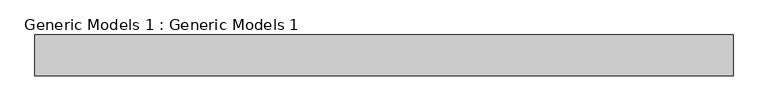
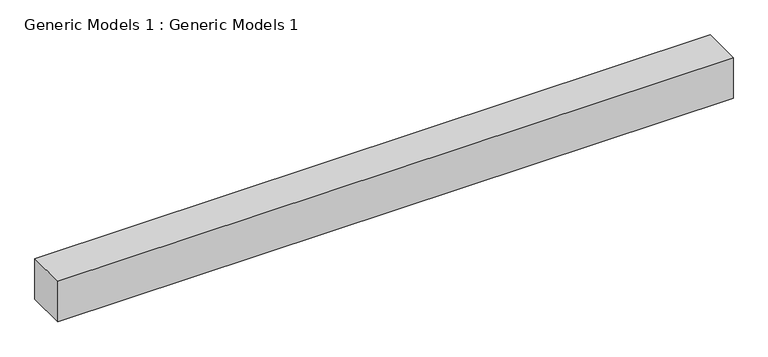
"""IFC4 building model written with IfcOpenShell, lengths in millimetres: proxy geometry, Generic Models 1 : Generic Models 1."""

from ifc_helpers import new_model, si_unit, frame, origin, place, context, project, spatial, polyline, outline, extrude, source, transform, mapped, element, save


def generic_models_1_generic_models_1_a2adb7c9(model_context):
    return source(origin(), model_context, "Body", "SweptSolid", [
        extrude(outline(polyline([(-12252.1280602, -5734.4090801), (-17444.0507021, -5734.4090801), (-17444.0507021, -5429.6090801), (-12252.1280602, -5429.6090801), (-12252.1280602, -5734.4090801)])), frame((0.0, 0.0, 5572.0), z_axis=(0.0, 0.0, 1.0), x_axis=(1.0, 0.0, 0.0)), (0.0, 0.0, 1.0), 330.2),
    ])


if __name__ == "__main__":
    model = new_model("IFC4")
    model_context = context("Model", 3, world=origin())
    ifc_project = project(units=[si_unit("LENGTHUNIT", "METRE", prefix="MILLI")], contexts=[model_context])
    site = spatial("IfcSite", under=ifc_project)
    building = spatial("IfcBuilding", under=site)
    placement = place(None, origin())
    generic_models_1_generic_models_1_shape = generic_models_1_generic_models_1_a2adb7c9(model_context)
    element("IfcBuildingElementProxy", 1, Name="Generic Models 1 : Generic Models 1", ObjectType="Generic Models 1 : Generic Models 1", at=placement, inside=building, context=model_context, shape_type="MappedRepresentation", body=[
        mapped(generic_models_1_generic_models_1_shape, transform((0.0, 0.0, 0.0), x_axis=(1.0, 0.0, 0.0), y_axis=(0.0, 1.0, 0.0), z_axis=(0.0, 0.0, 1.0))),
    ])
    save(model, "model.ifc")
